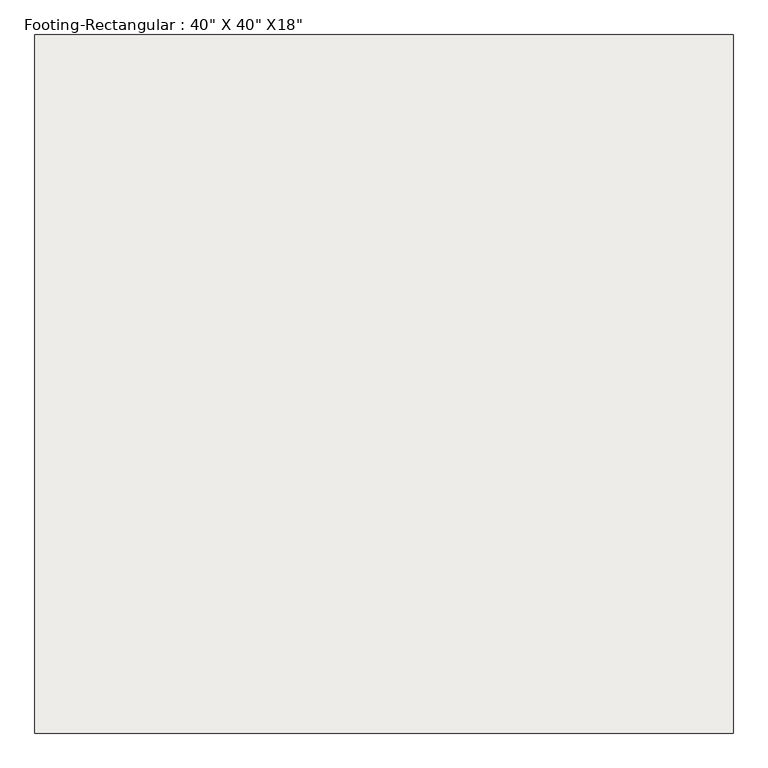
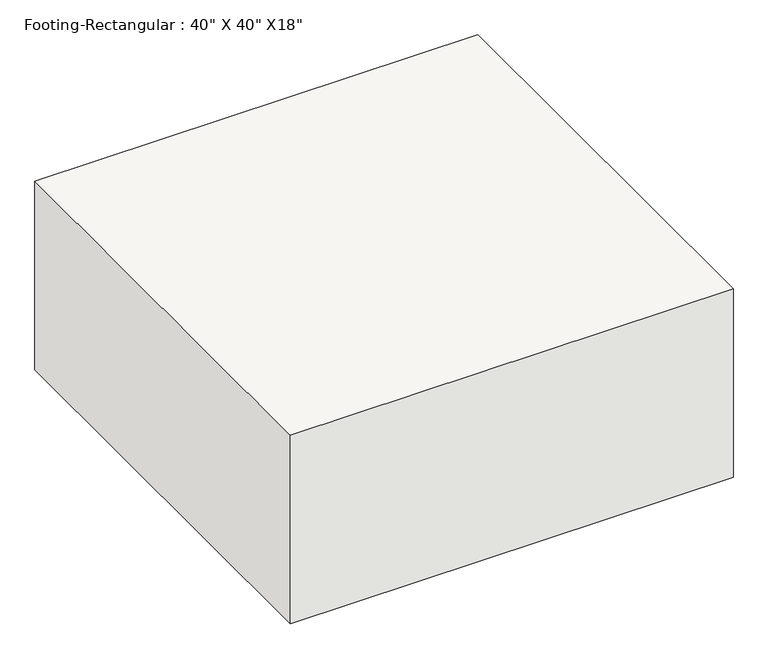
"""IFC4 building model written with IfcOpenShell, lengths in millimetres: slab geometry."""

from ifc_helpers import new_model, si_unit, frame, origin, place, context, project, spatial, polyline, outline, extrude, source, transform, mapped, element, save


def slab_21579c01(model_context):
    return source(origin(), model_context, "Body", "SweptSolid", [
        extrude(outline(polyline([(508.0, 508.0), (508.0, -508.0), (-508.0, -508.0), (-508.0, 508.0), (508.0, 508.0)])), frame((0.0, 0.0, -457.2), z_axis=(0.0, 0.0, 1.0), x_axis=(1.0, 0.0, 0.0)), (0.0, 0.0, 1.0), 457.2),
    ])


if __name__ == "__main__":
    model = new_model("IFC4")
    model_context = context("Model", 3, world=origin())
    ifc_project = project(units=[si_unit("LENGTHUNIT", "METRE", prefix="MILLI")], contexts=[model_context])
    site = spatial("IfcSite", under=ifc_project)
    building = spatial("IfcBuilding", under=site)
    placement = place(None, origin())
    slab_shape = slab_21579c01(model_context)
    element("IfcSlab", 1, ObjectType="Footing-Rectangular : 40\" X 40\" X18\"", at=placement, inside=building, context=model_context, shape_type="MappedRepresentation", body=[
        mapped(slab_shape, transform((0.0, 0.0, 0.0), x_axis=(1.0, 0.0, 0.0), y_axis=(0.0, 1.0, 0.0), z_axis=(0.0, 0.0, 1.0))),
    ])
    save(model, "model.ifc")

# Revit data of these elements
# Type "Footing-Rectangular : 40\" X 40\" X18\""
#   Assembly Code = "A1010100"
#   Width = 3' - 4"
#   Length = 3' - 4"
#   Foundation Thickness = 1' - 6"
#   Structural Material [instance default] = Concrete, Cast-in-Place gray
# Element 1 (IfcSlab, "Footing-Rectangular : 40\" X 40\" X18\"")
#   Materials on its faces: "Concrete, Cast-in-Place gray"
# Materials
#   "Concrete, Cast-in-Place gray": class "Concrete", colour RGB 192 192 192, transparency 0, Description = "Cast-in-place concrete", Cost = 0
